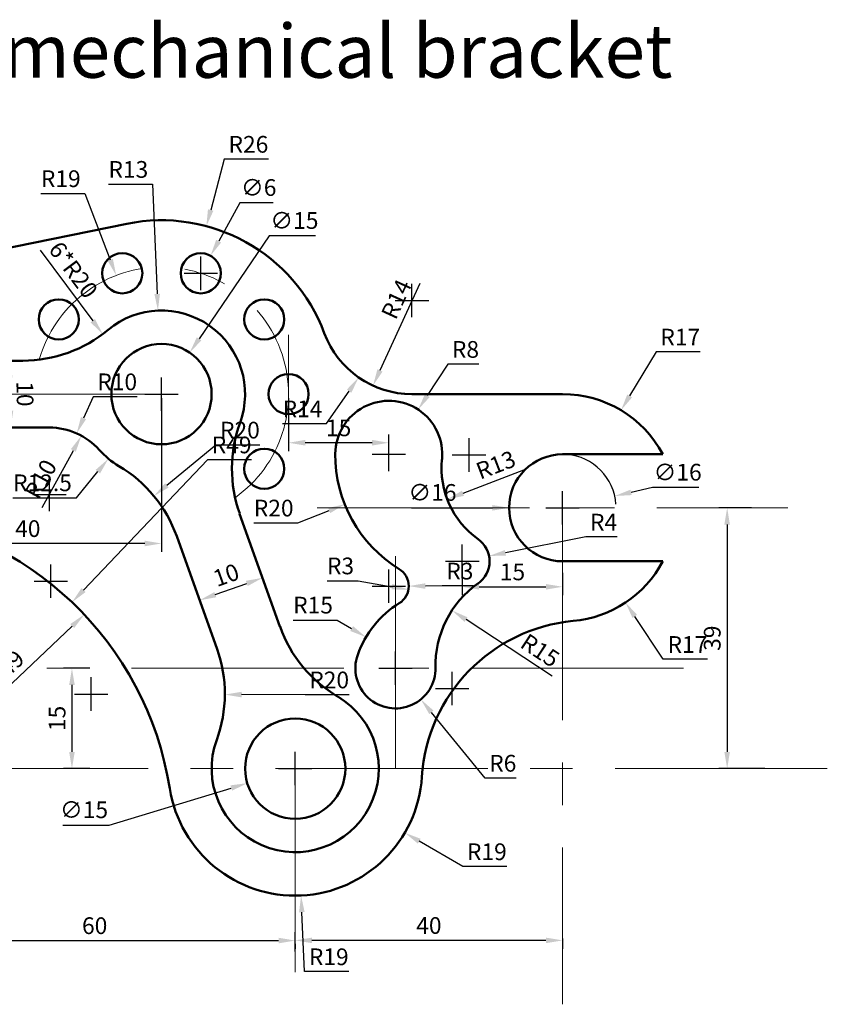
# Model space of a CAD drawing. Units: millimetres. Extents: x 59 to 241, y 36 to 183.
# Tile 2 of 2: x 120 to 241, y 36 to 183. Entities that reach past the tile are written whole.
import ezdxf

# ---------------------------------------------------------------- set-up
doc = ezdxf.new("R2010")
doc.units = ezdxf.units.MM
doc.linetypes.add('CENTER', pattern=[50.8, 31.75, -6.35, 6.35, -6.35])
for name, color, linetype, lineweight in [('M-CNTR', 1, 'CENTER', 18), ('M-DIMS', 2, 'Continuous', 25), ('M-OUTL', 7, 'Continuous', 50), ('M-TEXT', 3, 'Continuous', 25)]:
    doc.layers.add(name, color=color, linetype=linetype, lineweight=lineweight)
doc.styles.get("Standard").update_dxf_attribs({"font": 'arial.ttf'})
doc.dimstyles.new('ISO-25', dxfattribs={"dimtxt": 2.5, "dimasz": 2.5, "dimexe": 1.25, "dimexo": 0.625, "dimtad": 1, "dimtoh": 1, "dimdec": 0, "dimtxsty": 'Standard', "dimcen": 2.5, "dimadec": 0, "dimazin": 0, "dimtfac": 1, "dimtdec": 0, "dimtofl": 0, "dimtmove": 0, "dimatfit": 3, "dimfxl": 1, "dimarcsym": 0})

# ---------------------------------------------------------------- blocks, each defined once
blk = doc.blocks.new('*D2')
at = {"layer": 'Defpoints', "color": 0, "transparency": 16777216}
for p in [(101.46, 127.43), (161.46, 45.87), (161.46, 45.71)]:
    blk.add_point(p, dxfattribs=at)
at = {"layer": 'M-DIMS', "color": 0, "lineweight": -2, "transparency": 16777216}
for p, q in [((101.46, 126.8), (101.46, 44.46)), ((103.96, 45.71), (158.96, 45.71)), ((161.46, 45.24), (161.46, 44.46))]:
    blk.add_line(p, q, dxfattribs=at)
at = {"layer": 'M-DIMS', "color": 0, "transparency": 16777216}
for points in [[(103.96, 46.13), (103.96, 45.29), (101.46, 45.71)], [(158.96, 46.13), (158.96, 45.29), (161.46, 45.71)]]:
    blk.add_solid(points, dxfattribs=at)
at = {"layer": 'M-DIMS', "color": 0, "transparency": 16777216, "insert": (131.46, 47.61), "char_height": 2.5, "attachment_point": 5}
blk.add_mtext('60', dxfattribs=at)
blk = doc.blocks.new('*D3')
at = {"layer": 'Defpoints', "color": 0, "transparency": 16777216}
for p in [(161.46, 45.74), (201.46, 46.63), (161.46, 43.45)]:
    blk.add_point(p, dxfattribs=at)
at = {"layer": 'M-DIMS', "color": 0, "lineweight": -2, "transparency": 16777216}
for p, q in [((161.46, 44.07), (161.46, 46.99)), ((198.96, 45.74), (163.96, 45.74)), ((201.46, 46.01), (201.46, 44.49))]:
    blk.add_line(p, q, dxfattribs=at)
at = {"layer": 'M-DIMS', "color": 0, "transparency": 16777216}
for points in [[(163.96, 46.15), (163.96, 45.32), (161.46, 45.74)], [(198.96, 46.15), (198.96, 45.32), (201.46, 45.74)]]:
    blk.add_solid(points, dxfattribs=at)
at = {"layer": 'M-DIMS', "color": 0, "transparency": 16777216, "insert": (181.46, 47.64), "char_height": 2.5, "attachment_point": 5}
blk.add_mtext('40', dxfattribs=at)
blk = doc.blocks.new('*D4')
at = {"layer": 'Defpoints', "color": 0, "transparency": 16777216}
for p in [(209.26, 112.19), (193.65, 108.67)]:
    blk.add_point(p, dxfattribs=at)
at = {"layer": 'M-DIMS', "color": 0, "lineweight": -2, "transparency": 16777216}
for p, q in [((214.9, 113.46), (211.7, 112.73)), ((221.82, 113.46), (214.9, 113.46)), ((201.46, 107.93), (201.46, 112.93)), ((198.96, 110.43), (203.96, 110.43))]:
    blk.add_line(p, q, dxfattribs=at)
blk.add_arc((201.46, 110.43), 8, 3.7384, 85.5238, dxfattribs=at)
at = {"layer": 'M-DIMS', "color": 0, "transparency": 16777216}
blk.add_solid([(211.61, 113.14), (211.79, 112.33), (209.26, 112.19)], dxfattribs=at)
at = {"layer": 'M-DIMS', "color": 0, "transparency": 16777216, "insert": (218.67, 115.43), "char_height": 2.5, "attachment_point": 5}
blk.add_mtext('∅16', dxfattribs=at)
blk = doc.blocks.new('*D5')
at = {"layer": 'Defpoints', "color": 0, "transparency": 16777216}
for p in [(168.63, 73.61), (154.28, 69.25)]:
    blk.add_point(p, dxfattribs=at)
at = {"layer": 'M-DIMS', "color": 0, "lineweight": -2, "transparency": 16777216}
for p, q in [((161.46, 68.93), (161.46, 73.93)), ((158.96, 71.43), (163.96, 71.43)), ((133.65, 62.98), (151.89, 68.52)), ((126.71, 62.98), (133.65, 62.98))]:
    blk.add_line(p, q, dxfattribs=at)
at = {"layer": 'M-DIMS', "color": 0, "transparency": 16777216}
blk.add_solid([(151.77, 68.92), (152.01, 68.12), (154.28, 69.25)], dxfattribs=at)
at = {"layer": 'M-DIMS', "color": 0, "transparency": 16777216, "insert": (129.87, 64.95), "char_height": 2.5, "attachment_point": 5}
blk.add_mtext('∅15', dxfattribs=at)
blk = doc.blocks.new('*D6')
at = {"layer": 'Defpoints', "color": 0, "transparency": 16777216}
for p in [(148.79, 148.12), (145.87, 142.88)]:
    blk.add_point(p, dxfattribs=at)
at = {"layer": 'M-DIMS', "color": 0, "lineweight": -2, "transparency": 16777216}
for p, q in [((153.2, 156.03), (150.01, 150.3)), ((158.18, 156.03), (153.2, 156.03)), ((147.33, 143), (147.33, 148)), ((144.83, 145.5), (149.83, 145.5))]:
    blk.add_line(p, q, dxfattribs=at)
at = {"layer": 'M-DIMS', "color": 0, "transparency": 16777216}
blk.add_solid([(149.64, 150.51), (150.37, 150.1), (148.79, 148.12)], dxfattribs=at)
at = {"layer": 'M-DIMS', "color": 0, "transparency": 16777216, "insert": (156, 158), "char_height": 2.5, "attachment_point": 5}
blk.add_mtext('∅6', dxfattribs=at)
blk = doc.blocks.new('*D7')
at = {"layer": 'Defpoints', "color": 0, "transparency": 16777216}
for p in [(145.67, 133.63), (137.24, 121.23)]:
    blk.add_point(p, dxfattribs=at)
at = {"layer": 'M-DIMS', "color": 0, "lineweight": -2, "transparency": 16777216}
for p, q in [((157.55, 151.1), (147.08, 135.7)), ((164.5, 151.1), (157.55, 151.1)), ((141.46, 124.93), (141.46, 129.93)), ((138.96, 127.43), (143.96, 127.43))]:
    blk.add_line(p, q, dxfattribs=at)
at = {"layer": 'M-DIMS', "color": 0, "transparency": 16777216}
blk.add_solid([(146.74, 135.93), (147.42, 135.46), (145.67, 133.63)], dxfattribs=at)
at = {"layer": 'M-DIMS', "color": 0, "transparency": 16777216, "insert": (161.34, 153.07), "char_height": 2.5, "attachment_point": 5}
blk.add_mtext('∅15', dxfattribs=at)
blk = doc.blocks.new('*D8')
at = {"layer": 'Defpoints', "color": 0, "transparency": 16777216}
for p in [(120.69, 152.43), (132.67, 136.41)]:
    blk.add_point(p, dxfattribs=at)
at = {"layer": 'M-DIMS', "color": 0, "lineweight": -2, "transparency": 16777216}
blk.add_line((123.29, 148.95), (131.17, 138.41), dxfattribs=at)
at = {"layer": 'M-DIMS', "color": 0, "transparency": 16777216}
blk.add_solid([(131.5, 138.66), (130.84, 138.16), (132.67, 136.41)], dxfattribs=at)
at = {"layer": 'M-DIMS', "color": 0, "transparency": 16777216, "insert": (128.01, 145.82), "char_height": 2.5, "attachment_point": 5, "rotation": 306.7855}
blk.add_mtext('6*R20', dxfattribs=at)
blk = doc.blocks.new('*D11')
at = {"layer": 'Defpoints', "color": 0, "transparency": 16777216}
for p in [(129.47, 121.21), (124.69, 112.43)]:
    blk.add_point(p, dxfattribs=at)
at = {"layer": 'M-DIMS', "color": 0, "lineweight": -2, "transparency": 16777216}
blk.add_line((123.63, 110.48), (128.27, 119.02), dxfattribs=at)
at = {"layer": 'M-DIMS', "color": 0, "transparency": 16777216}
blk.add_solid([(127.91, 119.21), (128.64, 118.82), (129.47, 121.21)], dxfattribs=at)
at = {"layer": 'M-DIMS', "color": 0, "transparency": 16777216, "insert": (123.68, 114.56), "char_height": 2.5, "attachment_point": 5, "rotation": 61.439}
blk.add_mtext('R10', dxfattribs=at)
blk = doc.blocks.new('*D13')
at = {"layer": 'Defpoints', "color": 0, "transparency": 16777216}
for p in [(129.91, 94.46), (94.29, 60.81)]:
    blk.add_point(p, dxfattribs=at)
at = {"layer": 'M-DIMS', "color": 0, "lineweight": -2, "transparency": 16777216}
blk.add_line((117.07, 82.33), (128.09, 92.74), dxfattribs=at)
at = {"layer": 'M-DIMS', "color": 0, "transparency": 16777216}
blk.add_solid([(127.81, 93.05), (128.38, 92.44), (129.91, 94.46)], dxfattribs=at)
at = {"layer": 'M-DIMS', "color": 0, "transparency": 16777216, "insert": (118.39, 86.19), "char_height": 2.5, "attachment_point": 5, "rotation": 43.3695}
blk.add_mtext('R49', dxfattribs=at)
blk = doc.blocks.new('*D14')
at = {"layer": 'Defpoints', "color": 0, "transparency": 16777216}
for p in [(161.46, 71.43), (177.86, 61.83)]:
    blk.add_point(p, dxfattribs=at)
at = {"layer": 'M-DIMS', "color": 0, "lineweight": -2, "transparency": 16777216}
for p, q in [((161.46, 68.93), (161.46, 73.93)), ((158.96, 71.43), (163.96, 71.43)), ((186.52, 56.77), (180.02, 60.57)), ((193.12, 56.77), (186.52, 56.77))]:
    blk.add_line(p, q, dxfattribs=at)
at = {"layer": 'M-DIMS', "color": 0, "transparency": 16777216}
blk.add_solid([(180.23, 60.93), (179.81, 60.21), (177.86, 61.83)], dxfattribs=at)
at = {"layer": 'M-DIMS', "color": 0, "transparency": 16777216, "insert": (190.13, 58.67), "char_height": 2.5, "attachment_point": 5}
blk.add_mtext('R19', dxfattribs=at)
blk = doc.blocks.new('*D15')
at = {"layer": 'Defpoints', "color": 0, "transparency": 16777216}
for p in [(176.46, 86.43), (180.25, 81.78)]:
    blk.add_point(p, dxfattribs=at)
at = {"layer": 'M-DIMS', "color": 0, "lineweight": -2, "transparency": 16777216}
for p, q in [((176.46, 83.93), (176.46, 88.93)), ((173.96, 86.43), (178.96, 86.43)), ((189.87, 69.99), (181.83, 79.84)), ((194.52, 69.99), (189.87, 69.99))]:
    blk.add_line(p, q, dxfattribs=at)
at = {"layer": 'M-DIMS', "color": 0, "transparency": 16777216}
blk.add_solid([(182.15, 80.11), (181.51, 79.58), (180.25, 81.78)], dxfattribs=at)
at = {"layer": 'M-DIMS', "color": 0, "transparency": 16777216, "insert": (192.51, 71.9), "char_height": 2.5, "attachment_point": 5}
blk.add_mtext('R6', dxfattribs=at)
blk = doc.blocks.new('*D16')
at = {"layer": 'Defpoints', "color": 0, "transparency": 16777216}
for p in [(172.05, 91.09), (184.94, 83.42)]:
    blk.add_point(p, dxfattribs=at)
at = {"layer": 'M-DIMS', "color": 0, "lineweight": -2, "transparency": 16777216}
for p, q in [((161.14, 93.65), (167.75, 93.65)), ((167.75, 93.65), (169.9, 92.37)), ((184.94, 80.92), (184.94, 85.92)), ((182.44, 83.42), (187.44, 83.42))]:
    blk.add_line(p, q, dxfattribs=at)
at = {"layer": 'M-DIMS', "color": 0, "transparency": 16777216}
blk.add_solid([(170.11, 92.73), (169.69, 92.01), (172.05, 91.09)], dxfattribs=at)
at = {"layer": 'M-DIMS', "color": 0, "transparency": 16777216, "insert": (164.13, 95.55), "char_height": 2.5, "attachment_point": 5}
blk.add_mtext('R15', dxfattribs=at)
blk = doc.blocks.new('*D17')
at = {"layer": 'Defpoints', "color": 0, "transparency": 16777216}
for p in [(175.45, 98.71), (178.4, 98.19)]:
    blk.add_point(p, dxfattribs=at)
at = {"layer": 'M-DIMS', "color": 0, "lineweight": -2, "transparency": 16777216}
for p, q in [((166.22, 99.51), (170.88, 99.51)), ((170.88, 99.51), (175.94, 98.63))]:
    blk.add_line(p, q, dxfattribs=at)
at = {"layer": 'M-DIMS', "color": 0, "transparency": 16777216}
blk.add_solid([(176.01, 99.04), (175.87, 98.22), (178.4, 98.19)], dxfattribs=at)
at = {"layer": 'M-DIMS', "color": 0, "transparency": 16777216, "insert": (168.24, 101.41), "char_height": 2.5, "attachment_point": 5}
blk.add_mtext('R3', dxfattribs=at)
blk = doc.blocks.new('*D18')
at = {"layer": 'Defpoints', "color": 0, "transparency": 16777216}
for p in [(187.46, 118.33), (168.87, 110.95)]:
    blk.add_point(p, dxfattribs=at)
at = {"layer": 'M-DIMS', "color": 0, "lineweight": -2, "transparency": 16777216}
for p, q in [((187.46, 115.83), (187.46, 120.83)), ((184.96, 118.33), (189.96, 118.33)), ((161.85, 108.16), (166.54, 110.03)), ((155.26, 108.16), (161.85, 108.16))]:
    blk.add_line(p, q, dxfattribs=at)
at = {"layer": 'M-DIMS', "color": 0, "transparency": 16777216}
blk.add_solid([(166.39, 110.41), (166.7, 109.64), (168.87, 110.95)], dxfattribs=at)
at = {"layer": 'M-DIMS', "color": 0, "transparency": 16777216, "insert": (158.24, 110.06), "char_height": 2.5, "attachment_point": 5}
blk.add_mtext('R20', dxfattribs=at)
blk = doc.blocks.new('*D19')
at = {"layer": 'Defpoints', "color": 0, "transparency": 16777216}
for p in [(190.45, 103.22), (186.46, 102.43)]:
    blk.add_point(p, dxfattribs=at)
at = {"layer": 'M-DIMS', "color": 0, "lineweight": -2, "transparency": 16777216}
for p, q in [((204.95, 106.08), (192.9, 103.7)), ((209.6, 106.08), (204.95, 106.08)), ((186.46, 99.93), (186.46, 104.93)), ((183.96, 102.43), (188.96, 102.43))]:
    blk.add_line(p, q, dxfattribs=at)
at = {"layer": 'M-DIMS', "color": 0, "transparency": 16777216}
blk.add_solid([(192.82, 104.11), (192.98, 103.29), (190.45, 103.22)], dxfattribs=at)
at = {"layer": 'M-DIMS', "color": 0, "transparency": 16777216, "insert": (207.59, 107.96), "char_height": 2.5, "attachment_point": 5}
blk.add_mtext('R4', dxfattribs=at)
blk = doc.blocks.new('*D20')
at = {"layer": 'Defpoints', "color": 0, "transparency": 16777216}
for p in [(184.92, 95.08), (197.45, 86.85)]:
    blk.add_point(p, dxfattribs=at)
at = {"layer": 'M-DIMS', "color": 0, "lineweight": -2, "transparency": 16777216}
blk.add_line((199.9, 85.24), (187.01, 93.71), dxfattribs=at)
at = {"layer": 'M-DIMS', "color": 0, "transparency": 16777216}
blk.add_solid([(187.23, 94.06), (186.78, 93.36), (184.92, 95.08)], dxfattribs=at)
at = {"layer": 'M-DIMS', "color": 0, "transparency": 16777216, "insert": (197.92, 88.82), "char_height": 2.5, "attachment_point": 5, "rotation": 326.7033}
blk.add_mtext('R15', dxfattribs=at)
blk = doc.blocks.new('*D21')
at = {"layer": 'Defpoints', "color": 0, "transparency": 16777216}
for p in [(179.85, 125.12), (175.46, 118.43)]:
    blk.add_point(p, dxfattribs=at)
at = {"layer": 'M-DIMS', "color": 0, "lineweight": -2, "transparency": 16777216}
for p, q in [((184.29, 131.89), (181.22, 127.21)), ((188.95, 131.89), (184.29, 131.89)), ((175.46, 115.93), (175.46, 120.93)), ((172.96, 118.43), (177.96, 118.43))]:
    blk.add_line(p, q, dxfattribs=at)
at = {"layer": 'M-DIMS', "color": 0, "transparency": 16777216}
blk.add_solid([(180.87, 127.44), (181.57, 126.98), (179.85, 125.12)], dxfattribs=at)
at = {"layer": 'M-DIMS', "color": 0, "transparency": 16777216, "insert": (186.93, 133.79), "char_height": 2.5, "attachment_point": 5}
blk.add_mtext('R8', dxfattribs=at)
blk = doc.blocks.new('*D22')
at = {"layer": 'Defpoints', "color": 0, "transparency": 16777216}
for p in [(196.35, 116.34), (184.21, 111.7)]:
    blk.add_point(p, dxfattribs=at)
at = {"layer": 'M-DIMS', "color": 0, "lineweight": -2, "transparency": 16777216}
blk.add_line((195.63, 116.06), (186.54, 112.59), dxfattribs=at)
at = {"layer": 'M-DIMS', "color": 0, "transparency": 16777216}
blk.add_solid([(186.4, 112.98), (186.69, 112.21), (184.21, 111.7)], dxfattribs=at)
at = {"layer": 'M-DIMS', "color": 0, "transparency": 16777216, "insert": (191.58, 116.55), "char_height": 2.5, "attachment_point": 5, "rotation": 20.8827}
blk.add_mtext('R13', dxfattribs=at)
blk = doc.blocks.new('*D23')
at = {"layer": 'Defpoints', "color": 0, "transparency": 16777216}
for p in [(178.93, 141.43), (173.1, 128.7)]:
    blk.add_point(p, dxfattribs=at)
at = {"layer": 'M-DIMS', "color": 0, "lineweight": -2, "transparency": 16777216}
blk.add_line((180.1, 143.99), (174.14, 130.97), dxfattribs=at)
at = {"layer": 'M-DIMS', "color": 0, "transparency": 16777216}
blk.add_solid([(173.76, 131.15), (174.52, 130.8), (173.1, 128.7)], dxfattribs=at)
at = {"layer": 'M-DIMS', "color": 0, "transparency": 16777216, "insert": (176.89, 141.49), "char_height": 2.5, "attachment_point": 5, "rotation": 65.3862}
blk.add_mtext('R14', dxfattribs=at)
blk = doc.blocks.new('*D24')
at = {"layer": 'Defpoints', "color": 0, "transparency": 16777216}
for p in [(148.17, 152.55), (141.46, 127.43)]:
    blk.add_point(p, dxfattribs=at)
at = {"layer": 'M-DIMS', "color": 0, "lineweight": -2, "transparency": 16777216}
for p, q in [((150.85, 162.56), (148.82, 154.96)), ((157.44, 162.56), (150.85, 162.56)), ((141.46, 124.93), (141.46, 129.93)), ((138.96, 127.43), (143.96, 127.43))]:
    blk.add_line(p, q, dxfattribs=at)
at = {"layer": 'M-DIMS', "color": 0, "transparency": 16777216}
blk.add_solid([(148.41, 155.07), (149.22, 154.85), (148.17, 152.55)], dxfattribs=at)
at = {"layer": 'M-DIMS', "color": 0, "transparency": 16777216, "insert": (154.46, 164.46), "char_height": 2.5, "attachment_point": 5}
blk.add_mtext('R26', dxfattribs=at)
blk = doc.blocks.new('*D25')
at = {"layer": 'Defpoints', "color": 0, "transparency": 16777216}
for p in [(140.92, 139.92), (141.46, 127.43)]:
    blk.add_point(p, dxfattribs=at)
at = {"layer": 'M-DIMS', "color": 0, "lineweight": -2, "transparency": 16777216}
for p, q in [((133.51, 158.81), (140.11, 158.81)), ((140.11, 158.81), (140.81, 142.41)), ((141.46, 124.93), (141.46, 129.93)), ((138.96, 127.43), (143.96, 127.43))]:
    blk.add_line(p, q, dxfattribs=at)
at = {"layer": 'M-DIMS', "color": 0, "transparency": 16777216}
blk.add_solid([(141.23, 142.43), (140.4, 142.4), (140.92, 139.92)], dxfattribs=at)
at = {"layer": 'M-DIMS', "color": 0, "transparency": 16777216, "insert": (136.5, 160.71), "char_height": 2.5, "attachment_point": 5}
blk.add_mtext('R13', dxfattribs=at)
blk = doc.blocks.new('*D26')
at = {"layer": 'Defpoints', "color": 0, "transparency": 16777216}
for p in [(134.68, 145.18), (141.46, 127.43)]:
    blk.add_point(p, dxfattribs=at)
at = {"layer": 'M-DIMS', "color": 0, "lineweight": -2, "transparency": 16777216}
for p, q in [((123.4, 157.42), (130.01, 157.42)), ((130.01, 157.42), (133.79, 147.51)), ((141.46, 124.93), (141.46, 129.93)), ((138.96, 127.43), (143.96, 127.43))]:
    blk.add_line(p, q, dxfattribs=at)
at = {"layer": 'M-DIMS', "color": 0, "transparency": 16777216}
blk.add_solid([(134.18, 147.66), (133.4, 147.37), (134.68, 145.18)], dxfattribs=at)
at = {"layer": 'M-DIMS', "color": 0, "transparency": 16777216, "insert": (126.39, 159.32), "char_height": 2.5, "attachment_point": 5}
blk.add_mtext('R19', dxfattribs=at)
blk = doc.blocks.new('*D27')
at = {"layer": 'Defpoints', "color": 0, "transparency": 16777216}
for p in [(141.46, 127.43), (101.46, 105.09), (101.46, 101.65)]:
    blk.add_point(p, dxfattribs=at)
at = {"layer": 'M-DIMS', "color": 0, "lineweight": -2, "transparency": 16777216}
for p, q in [((141.46, 126.8), (141.46, 103.84)), ((101.46, 102.27), (101.46, 106.34)), ((138.96, 105.09), (103.96, 105.09))]:
    blk.add_line(p, q, dxfattribs=at)
at = {"layer": 'M-DIMS', "color": 0, "transparency": 16777216}
for points in [[(103.96, 105.51), (103.96, 104.68), (101.46, 105.09)], [(138.96, 105.51), (138.96, 104.68), (141.46, 105.09)]]:
    blk.add_solid(points, dxfattribs=at)
at = {"layer": 'M-DIMS', "color": 0, "transparency": 16777216, "insert": (121.46, 106.99), "char_height": 2.5, "attachment_point": 5}
blk.add_mtext('40', dxfattribs=at)
blk = doc.blocks.new('*D28')
at = {"layer": 'Defpoints', "color": 0, "transparency": 16777216}
for p in [(156.55, 100.04), (156.58, 99.96), (147.13, 96.68)]:
    blk.add_point(p, dxfattribs=at)
at = {"layer": 'M-DIMS', "color": 0, "lineweight": -2, "transparency": 16777216}
for p, q in [((149.51, 97.44), (154.22, 99.12)), ((156.76, 99.45), (157, 98.78)), ((147.34, 96.09), (147.58, 95.42))]:
    blk.add_line(p, q, dxfattribs=at)
at = {"layer": 'M-DIMS', "color": 0, "transparency": 16777216}
for points in [[(154.08, 99.51), (154.36, 98.73), (156.58, 99.96)], [(149.37, 97.83), (149.65, 97.05), (147.16, 96.6)]]:
    blk.add_solid(points, dxfattribs=at)
at = {"layer": 'M-DIMS', "color": 0, "transparency": 16777216, "insert": (151.23, 100.07), "char_height": 2.5, "attachment_point": 5, "rotation": 19.6538}
blk.add_mtext('10', dxfattribs=at)
blk = doc.blocks.new('*D29')
at = {"layer": 'Defpoints', "color": 0, "transparency": 16777216}
for p in [(118.72, 132.43), (118.9, 122.43), (118.9, 122.43)]:
    blk.add_point(p, dxfattribs=at)
at = {"layer": 'M-DIMS', "color": 0, "lineweight": -2, "transparency": 16777216}
for p, q in [((119.35, 132.44), (119.97, 132.45)), ((118.77, 129.93), (118.86, 124.93)), ((119.53, 122.44), (120.15, 122.45))]:
    blk.add_line(p, q, dxfattribs=at)
at = {"layer": 'M-DIMS', "color": 0, "transparency": 16777216}
for points in [[(119.18, 129.94), (118.35, 129.92), (118.72, 132.43)], [(119.28, 124.94), (118.44, 124.92), (118.9, 122.43)]]:
    blk.add_solid(points, dxfattribs=at)
at = {"layer": 'M-DIMS', "color": 0, "transparency": 16777216, "insert": (120.71, 127.46), "char_height": 2.5, "attachment_point": 5, "rotation": 271.0391}
blk.add_mtext('10', dxfattribs=at)
blk = doc.blocks.new('*D30')
at = {"layer": 'Defpoints', "color": 0, "transparency": 16777216}
for p in [(131.34, 86.43), (128.06, 71.43), (131.34, 71.43)]:
    blk.add_point(p, dxfattribs=at)
at = {"layer": 'M-DIMS', "color": 0, "lineweight": -2, "transparency": 16777216}
for p, q in [((130.72, 86.43), (126.81, 86.43)), ((128.06, 83.93), (128.06, 73.93)), ((130.72, 71.43), (126.81, 71.43))]:
    blk.add_line(p, q, dxfattribs=at)
at = {"layer": 'M-DIMS', "color": 0, "transparency": 16777216}
for points in [[(127.64, 83.93), (128.48, 83.93), (128.06, 86.43)], [(127.64, 73.93), (128.48, 73.93), (128.06, 71.43)]]:
    blk.add_solid(points, dxfattribs=at)
at = {"layer": 'M-DIMS', "color": 0, "transparency": 16777216, "insert": (126.16, 78.93), "char_height": 2.5, "attachment_point": 5, "rotation": 90}
blk.add_mtext('15', dxfattribs=at)
blk = doc.blocks.new('*D31')
at = {"layer": 'Defpoints', "color": 0, "transparency": 16777216}
for p in [(186.46, 102.43), (201.46, 101.33), (201.46, 98.62)]:
    blk.add_point(p, dxfattribs=at)
at = {"layer": 'M-DIMS', "color": 0, "lineweight": -2, "transparency": 16777216}
for p, q in [((186.46, 101.8), (186.46, 97.37)), ((201.46, 100.71), (201.46, 97.37)), ((188.96, 98.62), (198.96, 98.62))]:
    blk.add_line(p, q, dxfattribs=at)
at = {"layer": 'M-DIMS', "color": 0, "transparency": 16777216}
for points in [[(188.96, 99.03), (188.96, 98.2), (186.46, 98.62)], [(198.96, 99.03), (198.96, 98.2), (201.46, 98.62)]]:
    blk.add_solid(points, dxfattribs=at)
at = {"layer": 'M-DIMS', "color": 0, "transparency": 16777216, "insert": (193.96, 100.52), "char_height": 2.5, "attachment_point": 5}
blk.add_mtext('15', dxfattribs=at)
blk = doc.blocks.new('*D32')
at = {"layer": 'Defpoints', "color": 0, "transparency": 16777216}
for p in [(160.46, 127.43), (160.46, 120.16), (175.46, 118.43)]:
    blk.add_point(p, dxfattribs=at)
at = {"layer": 'M-DIMS', "color": 0, "lineweight": -2, "transparency": 16777216}
for p, q in [((160.46, 126.8), (160.46, 118.91)), ((175.46, 119.05), (175.46, 121.41)), ((172.96, 120.16), (162.96, 120.16))]:
    blk.add_line(p, q, dxfattribs=at)
at = {"layer": 'M-DIMS', "color": 0, "transparency": 16777216}
for points in [[(162.96, 120.58), (162.96, 119.74), (160.46, 120.16)], [(172.96, 120.58), (172.96, 119.74), (175.46, 120.16)]]:
    blk.add_solid(points, dxfattribs=at)
at = {"layer": 'M-DIMS', "color": 0, "transparency": 16777216, "insert": (167.96, 122.06), "char_height": 2.5, "attachment_point": 5}
blk.add_mtext('15', dxfattribs=at)
blk = doc.blocks.new('*D33')
at = {"layer": 'Defpoints', "color": 0, "transparency": 16777216}
for p in [(230.32, 110.43), (226.08, 71.43), (232.34, 71.43)]:
    blk.add_point(p, dxfattribs=at)
at = {"layer": 'M-DIMS', "color": 0, "lineweight": -2, "transparency": 16777216}
for p, q in [((229.7, 110.43), (224.83, 110.43)), ((226.08, 107.93), (226.08, 73.93)), ((231.71, 71.43), (224.83, 71.43))]:
    blk.add_line(p, q, dxfattribs=at)
at = {"layer": 'M-DIMS', "color": 0, "transparency": 16777216}
for points in [[(225.66, 107.93), (226.49, 107.93), (226.08, 110.43)], [(225.66, 73.93), (226.49, 73.93), (226.08, 71.43)]]:
    blk.add_solid(points, dxfattribs=at)
at = {"layer": 'M-DIMS', "color": 0, "transparency": 16777216, "insert": (224.17, 90.93), "char_height": 2.5, "attachment_point": 5, "rotation": 90}
blk.add_mtext('39', dxfattribs=at)
blk = doc.blocks.new('*D34')
at = {"layer": 'Defpoints', "color": 0, "transparency": 16777216}
for p in [(128.07, 96.31), (94.29, 60.81)]:
    blk.add_point(p, dxfattribs=at)
at = {"layer": 'M-DIMS', "color": 0, "lineweight": -2, "transparency": 16777216}
for p, q in [((148.34, 117.61), (129.79, 98.12)), ((154.94, 117.61), (148.34, 117.61)), ((94.29, 58.31), (94.29, 63.31)), ((91.79, 60.81), (96.79, 60.81))]:
    blk.add_line(p, q, dxfattribs=at)
at = {"layer": 'M-DIMS', "color": 0, "transparency": 16777216}
blk.add_solid([(129.49, 98.41), (130.1, 97.83), (128.07, 96.31)], dxfattribs=at)
at = {"layer": 'M-DIMS', "color": 0, "transparency": 16777216, "insert": (151.95, 119.51), "char_height": 2.5, "attachment_point": 5}
blk.add_mtext('R49', dxfattribs=at)
blk = doc.blocks.new('*D35')
at = {"layer": 'Defpoints', "color": 0, "transparency": 16777216}
for p in [(130.93, 82.58), (150.93, 82.5)]:
    blk.add_point(p, dxfattribs=at)
at = {"layer": 'M-DIMS', "color": 0, "lineweight": -2, "transparency": 16777216}
for p, q in [((130.93, 80.08), (130.93, 85.08)), ((128.43, 82.58), (133.43, 82.58)), ((162.93, 82.46), (153.43, 82.5)), ((169.52, 82.46), (162.93, 82.46))]:
    blk.add_line(p, q, dxfattribs=at)
at = {"layer": 'M-DIMS', "color": 0, "transparency": 16777216}
blk.add_solid([(153.43, 82.91), (153.43, 82.08), (150.93, 82.5)], dxfattribs=at)
at = {"layer": 'M-DIMS', "color": 0, "transparency": 16777216, "insert": (166.54, 84.36), "char_height": 2.5, "attachment_point": 5}
blk.add_mtext('R20', dxfattribs=at)
blk = doc.blocks.new('*D36')
at = {"layer": 'Defpoints', "color": 0, "transparency": 16777216}
for p in [(140.33, 112.19), (124.9, 99.46)]:
    blk.add_point(p, dxfattribs=at)
at = {"layer": 'M-DIMS', "color": 0, "lineweight": -2, "transparency": 16777216}
for p, q in [((149.59, 119.82), (142.26, 113.78)), ((156.18, 119.82), (149.59, 119.82)), ((124.9, 96.96), (124.9, 101.96)), ((122.4, 99.46), (127.4, 99.46))]:
    blk.add_line(p, q, dxfattribs=at)
at = {"layer": 'M-DIMS', "color": 0, "transparency": 16777216}
blk.add_solid([(141.99, 114.1), (142.52, 113.46), (140.33, 112.19)], dxfattribs=at)
at = {"layer": 'M-DIMS', "color": 0, "transparency": 16777216, "insert": (153.19, 121.72), "char_height": 2.5, "attachment_point": 5}
blk.add_mtext('R20', dxfattribs=at)
blk = doc.blocks.new('*D37')
at = {"layer": 'Defpoints', "color": 0, "transparency": 16777216}
for p in [(161.46, 71.43), (162.34, 52.45)]:
    blk.add_point(p, dxfattribs=at)
at = {"layer": 'M-DIMS', "color": 0, "lineweight": -2, "transparency": 16777216}
for p, q in [((161.46, 68.93), (161.46, 73.93)), ((158.96, 71.43), (163.96, 71.43)), ((162.87, 41.06), (162.45, 49.95)), ((169.47, 41.06), (162.87, 41.06))]:
    blk.add_line(p, q, dxfattribs=at)
at = {"layer": 'M-DIMS', "color": 0, "transparency": 16777216}
blk.add_solid([(162.87, 49.97), (162.04, 49.93), (162.34, 52.45)], dxfattribs=at)
at = {"layer": 'M-DIMS', "color": 0, "transparency": 16777216, "insert": (166.48, 42.96), "char_height": 2.5, "attachment_point": 5}
blk.add_mtext('R19', dxfattribs=at)
blk = doc.blocks.new('*D39')
at = {"layer": 'Defpoints', "color": 0, "transparency": 16777216}
for p in [(210.2, 125.01), (201.46, 110.43)]:
    blk.add_point(p, dxfattribs=at)
at = {"layer": 'M-DIMS', "color": 0, "lineweight": -2, "transparency": 16777216}
for p, q in [((215.45, 133.75), (211.49, 127.15)), ((222.05, 133.75), (215.45, 133.75)), ((201.46, 107.93), (201.46, 112.93)), ((198.96, 110.43), (203.96, 110.43))]:
    blk.add_line(p, q, dxfattribs=at)
at = {"layer": 'M-DIMS', "color": 0, "transparency": 16777216}
blk.add_solid([(211.13, 127.36), (211.85, 126.93), (210.2, 125.01)], dxfattribs=at)
at = {"layer": 'M-DIMS', "color": 0, "transparency": 16777216, "insert": (219.06, 135.63), "char_height": 2.5, "attachment_point": 5}
blk.add_mtext('R17', dxfattribs=at)
blk = doc.blocks.new('*D40')
at = {"layer": 'Defpoints', "color": 0, "transparency": 16777216}
for p in [(201.46, 110.43), (210.87, 96.27)]:
    blk.add_point(p, dxfattribs=at)
at = {"layer": 'M-DIMS', "color": 0, "lineweight": -2, "transparency": 16777216}
for p, q in [((201.46, 107.93), (201.46, 112.93)), ((198.96, 110.43), (203.96, 110.43)), ((216.52, 87.78), (212.26, 94.19)), ((223.12, 87.78), (216.52, 87.78))]:
    blk.add_line(p, q, dxfattribs=at)
at = {"layer": 'M-DIMS', "color": 0, "transparency": 16777216}
blk.add_solid([(212.61, 94.42), (211.91, 93.96), (210.87, 96.27)], dxfattribs=at)
at = {"layer": 'M-DIMS', "color": 0, "transparency": 16777216, "insert": (220.14, 89.66), "char_height": 2.5, "attachment_point": 5}
blk.add_mtext('R17', dxfattribs=at)
blk = doc.blocks.new('*D41')
at = {"layer": 'Defpoints', "color": 0, "transparency": 16777216}
for p in [(178.93, 141.43), (170.95, 129.93)]:
    blk.add_point(p, dxfattribs=at)
at = {"layer": 'M-DIMS', "color": 0, "lineweight": -2, "transparency": 16777216}
for p, q in [((178.93, 138.93), (178.93, 143.93)), ((176.43, 141.43), (181.43, 141.43)), ((166.16, 123.02), (169.52, 127.87)), ((159.57, 123.02), (166.16, 123.02))]:
    blk.add_line(p, q, dxfattribs=at)
at = {"layer": 'M-DIMS', "color": 0, "transparency": 16777216}
blk.add_solid([(169.18, 128.11), (169.86, 127.63), (170.95, 129.93)], dxfattribs=at)
at = {"layer": 'M-DIMS', "color": 0, "transparency": 16777216, "insert": (162.55, 124.9), "char_height": 2.5, "attachment_point": 5}
blk.add_mtext('R14', dxfattribs=at)
blk = doc.blocks.new('*D42')
at = {"layer": 'Defpoints', "color": 0, "transparency": 16777216}
for p in [(141.46, 127.43), (133.52, 117.77)]:
    blk.add_point(p, dxfattribs=at)
at = {"layer": 'M-DIMS', "color": 0, "lineweight": -2, "transparency": 16777216}
for p, q in [((141.46, 124.93), (141.46, 129.93)), ((138.96, 127.43), (143.96, 127.43)), ((128.73, 111.94), (131.94, 115.84)), ((119.2, 111.94), (128.73, 111.94))]:
    blk.add_line(p, q, dxfattribs=at)
at = {"layer": 'M-DIMS', "color": 0, "transparency": 16777216}
blk.add_solid([(131.61, 116.1), (132.26, 115.57), (133.52, 117.77)], dxfattribs=at)
at = {"layer": 'M-DIMS', "color": 0, "transparency": 16777216, "insert": (123.65, 113.84), "char_height": 2.5, "attachment_point": 5}
blk.add_mtext('R12.5', dxfattribs=at)
blk = doc.blocks.new('*D44')
at = {"layer": 'Defpoints', "color": 0, "transparency": 16777216}
for p in [(128.77, 121.56), (124.69, 112.43)]:
    blk.add_point(p, dxfattribs=at)
at = {"layer": 'M-DIMS', "color": 0, "lineweight": -2, "transparency": 16777216}
for p, q in [((131.22, 127.03), (129.79, 123.84)), ((137.81, 127.03), (131.22, 127.03)), ((124.69, 109.93), (124.69, 114.93)), ((122.19, 112.43), (127.19, 112.43))]:
    blk.add_line(p, q, dxfattribs=at)
at = {"layer": 'M-DIMS', "color": 0, "transparency": 16777216}
blk.add_solid([(129.41, 124.01), (130.17, 123.67), (128.77, 121.56)], dxfattribs=at)
at = {"layer": 'M-DIMS', "color": 0, "transparency": 16777216, "insert": (134.83, 128.94), "char_height": 2.5, "attachment_point": 5}
blk.add_mtext('R10', dxfattribs=at)
blk = doc.blocks.new('*D46')
at = {"layer": 'Defpoints', "color": 0, "transparency": 16777216}
for p in [(175.45, 98.71), (178.45, 98.72)]:
    blk.add_point(p, dxfattribs=at)
at = {"layer": 'M-DIMS', "color": 0, "lineweight": -2, "transparency": 16777216}
for p, q in [((175.45, 96.21), (175.45, 101.21)), ((172.95, 98.71), (177.95, 98.71)), ((183.45, 98.74), (180.95, 98.73)), ((188.1, 98.74), (183.45, 98.74))]:
    blk.add_line(p, q, dxfattribs=at)
at = {"layer": 'M-DIMS', "color": 0, "transparency": 16777216}
blk.add_solid([(180.95, 99.15), (180.95, 98.31), (178.45, 98.72)], dxfattribs=at)
at = {"layer": 'M-DIMS', "color": 0, "transparency": 16777216, "insert": (186.09, 100.64), "char_height": 2.5, "attachment_point": 5}
blk.add_mtext('R3', dxfattribs=at)
blk = doc.blocks.new('*D47')
at = {"layer": 'Defpoints', "color": 0, "transparency": 16777216}
for p in [(193.46, 110.43), (209.46, 110.43)]:
    blk.add_point(p, dxfattribs=at)
at = {"layer": 'M-DIMS', "color": 0, "lineweight": -2, "transparency": 16777216}
for p, q in [((201.46, 107.93), (201.46, 112.93)), ((178.84, 110.43), (185.77, 110.43)), ((185.77, 110.43), (190.96, 110.43)), ((198.96, 110.43), (203.96, 110.43))]:
    blk.add_line(p, q, dxfattribs=at)
at = {"layer": 'M-DIMS', "color": 0, "transparency": 16777216}
blk.add_solid([(190.96, 110.84), (190.96, 110.01), (193.46, 110.43)], dxfattribs=at)
at = {"layer": 'M-DIMS', "color": 0, "transparency": 16777216, "insert": (181.99, 112.4), "char_height": 2.5, "attachment_point": 5}
blk.add_mtext('∅16', dxfattribs=at)

msp = doc.modelspace()

# ---------------------------------------------------------------- linework, layer by layer
at = {"layer": 'M-CNTR'}
for p, q in [((160.46, 127.43), (160.46, 136.28)), ((141.46, 127.43), (69.53, 127.43)), ((164.75, 110.43), (235.16, 110.43)), ((201.46, 110.43), (201.46, 36.18)), ((176.46, 71.43), (176.46, 104.6)), ((219.53, 86.43), (115.15, 86.43)), ((241.06, 71.43), (65.85, 71.43)), ((161.46, 71.43), (161.46, 40.98))]:
    msp.add_line(p, q, dxfattribs=at)
msp.add_arc((141.46, 127.43), 19, 305.394, 164.2598, dxfattribs=at)
at = {"layer": 'M-OUTL'}
for p, q in [((136.26, 152.9), (97.86, 145.06)), ((113.12, 132.43), (120.69, 132.43)), ((201.46, 127.43), (178.93, 127.43)), ((113.12, 122.43), (124.69, 122.43)), ((201.46, 118.43), (216.46, 118.43)), ((153.15, 109.55), (159.18, 92.67)), ((143.73, 106.19), (149.77, 89.3)), ((201.46, 102.43), (216.46, 102.43))]:
    msp.add_line(p, q, dxfattribs=at)
for centre, radius in [((135.59, 145.5), 3), ((147.33, 145.5), 3), ((126.09, 138.6), 3), ((156.83, 138.6), 3), ((141.46, 127.43), 7.5), ((160.46, 127.43), 3), ((156.83, 116.26), 3), ((161.46, 71.43), 7.5)]:
    msp.add_circle(centre, radius, dxfattribs=at)
for centre, radius, start, end in [((141.46, 127.43), 26, 20.4873, 101.537), ((141.46, 127.43), 12.5, 339.9387, 129.7151), ((120.69, 152.43), 20, 270, 309.7151), ((178.93, 141.43), 14, 200.4873, 270), ((201.46, 110.43), 17, 28.0725, 90), ((175.46, 118.43), 8, 354.2856, 179.5159), ((124.69, 112.43), 10, 41.8103, 90), ((171.99, 116.28), 20, 159.9387, 199.6538), ((141.46, 127.43), 12.5, 221.8103, 239.369), ((187.46, 118.33), 20, 179.5159, 238.5198), ((201.46, 110.43), 8, 90, 270), ((124.9, 99.46), 20, 19.6538, 59.369), ((196.35, 116.34), 13, 174.2856, 234.5699), ((94.29, 60.81), 49, 8.9813, 83.8599), ((186.46, 102.43), 4.07, 305.2119, 54.5699), ((201.46, 110.43), 17, 275.3413, 331.9275), ((175.45, 98.71), 3, 301.8293, 58.5198), ((197.45, 86.85), 15, 125.2119, 181.602), ((184.94, 83.42), 15, 121.8293, 160.4648), ((205.37, 68.61), 25, 95.3413, 176.3284), ((178.02, 99.39), 20, 199.6538, 239.369), ((130.93, 82.58), 20, 339.9387, 19.6538), ((176.46, 86.43), 6, 160.4648, 1.1442), ((161.46, 71.43), 12.5, 159.9387, 59.369), ((161.46, 71.43), 19, 188.9813, 356.3284)]:
    msp.add_arc(centre, radius, start, end, dxfattribs=at)

# ---------------------------------------------------------------- texts
at = {"layer": 'M-TEXT', "insert": (71.54, 182.74), "char_height": 8, "attachment_point": 1}
msp.add_mtext_dynamic_manual_height_columns('complex mechanical bracket', width=206.9654, gutter_width=12.5, heights=[0], dxfattribs=at)

# ---------------------------------------------------------------- dimensions: what is measured, and where the dimension line sits
at = {"layer": 'M-DIMS'}
for center, mpoint, override, picture, middle in [((141.46, 127.43), (148.17, 152.55), {"dimclrd": 0, "dimclre": 0, "dimclrt": 0}, '*D24', (154.46, 162.56)), ((141.46, 127.43), (140.92, 139.92), {"dimclrd": 0, "dimclre": 0, "dimclrt": 0}, '*D25', (136.5, 158.81)), ((141.46, 127.43), (134.68, 145.18), {"dimclrd": 0, "dimclre": 0, "dimclrt": 0}, '*D26', (126.39, 157.42)), ((178.93, 141.43), (173.1, 128.7), {"dimclrd": 0, "dimclre": 0, "dimclrt": 0}, '*D23', (178.6, 140.71)), ((178.93, 141.43), (170.95, 129.93), {"dimdec": 0, "dimlfac": 1, "dimrnd": 0, "dimzin": 0, "dimdsep": 46, "dimlunit": 2}, '*D41', (162.55, 123.02)), ((201.46, 110.43), (210.2, 125.01), {"dimdec": 0, "dimlfac": 1, "dimrnd": 0, "dimzin": 0, "dimdsep": 46, "dimlunit": 2}, '*D39', (219.06, 133.75)), ((175.46, 118.43), (179.85, 125.12), {"dimclrd": 0, "dimclre": 0, "dimclrt": 0}, '*D21', (186.93, 131.89)), ((124.69, 112.43), (128.77, 121.56), {"dimdec": 0, "dimlfac": 1, "dimrnd": 0, "dimzin": 0, "dimdsep": 46, "dimlunit": 2}, '*D44', (134.83, 127.03)), ((124.9, 99.46), (140.33, 112.19), {"dimdec": 0, "dimlfac": 1, "dimrnd": 0, "dimzin": 0, "dimdsep": 46, "dimlunit": 2}, '*D36', (153.19, 119.82)), ((94.29, 60.81), (128.07, 96.31), {"dimdec": 0, "dimlfac": 1, "dimrnd": 0, "dimzin": 0, "dimdsep": 46, "dimlunit": 2}, '*D34', (151.95, 117.61)), ((124.69, 112.43), (129.47, 121.21), {"dimclrd": 0, "dimclre": 0, "dimclrt": 0}, '*D11', (125.35, 113.65)), ((196.35, 116.34), (184.21, 111.7), {"dimclrd": 0, "dimclre": 0, "dimclrt": 0}, '*D22', (192.25, 114.77)), ((201.46, 110.43), (210.87, 96.27), {"dimdec": 0, "dimlfac": 1, "dimrnd": 0, "dimzin": 0, "dimdsep": 46, "dimlunit": 2}, '*D40', (220.14, 87.78)), ((186.46, 102.43), (190.45, 103.22), {"dimclrd": 0, "dimclre": 0, "dimclrt": 0}, '*D19', (204.95, 106.08)), ((175.45, 98.71), (178.4, 98.19), {"dimclrd": 0, "dimclre": 0, "dimclrt": 0}, '*D17', (170.88, 99.51)), ((94.29, 60.81), (129.91, 94.46), {"dimclrd": 0, "dimclre": 0, "dimclrt": 0}, '*D13', (119.7, 84.81)), ((197.45, 86.85), (184.92, 95.08), {"dimclrd": 0, "dimclre": 0, "dimclrt": 0}, '*D20', (196.87, 87.23)), ((176.46, 86.43), (180.25, 81.78), {"dimclrd": 0, "dimclre": 0, "dimclrt": 0}, '*D15', (192.51, 69.99)), ((130.93, 82.58), (150.93, 82.5), {"dimdec": 0, "dimlfac": 1, "dimrnd": 0, "dimzin": 0, "dimdsep": 46, "dimlunit": 2}, '*D35', (162.93, 82.46)), ((161.46, 71.43), (177.86, 61.83), {"dimclrd": 0, "dimclre": 0, "dimclrt": 0}, '*D14', (190.13, 56.77)), ((161.46, 71.43), (162.34, 52.45), {"dimdec": 0, "dimlfac": 1, "dimrnd": 0, "dimzin": 0, "dimdsep": 46, "dimlunit": 2}, '*D37', (166.48, 41.06))]:
    dim = msp.add_radius_dim(center=center, mpoint=mpoint, dimstyle='ISO-25', override=override, dxfattribs=at)
    dim.commit()
    dim.dimension.update_dxf_attribs({"geometry": picture, "text_midpoint": middle, "dimtype": 164})
for p1, p2, picture, middle in [((145.87, 142.88), (148.79, 148.12), '*D6', (156, 156.03)), ((137.24, 121.23), (145.67, 133.63), '*D7', (161.34, 151.1)), ((193.65, 108.67), (209.26, 112.19), '*D4', (214.9, 113.46)), ((168.63, 73.61), (154.28, 69.25), '*D5', (129.87, 62.98))]:
    dim = msp.add_diameter_dim_2p(p1=p1, p2=p2, dimstyle='ISO-25', override={"dimclrd": 0, "dimclre": 0, "dimclrt": 0}, dxfattribs=at)
    dim.commit()
    dim.dimension.update_dxf_attribs({"geometry": picture, "text_midpoint": middle, "dimtype": 163})
dim = msp.add_radius_dim(center=(120.69, 152.43), mpoint=(132.67, 136.41), text='6*<>', dimstyle='ISO-25', override={"dimclrd": 0, "dimclre": 0, "dimclrt": 0}, dxfattribs=at)
dim.commit()
dim.dimension.update_dxf_attribs({"geometry": '*D8', "text_midpoint": (126.48, 144.68), "dimtype": 164})
for p1, p2, distance, picture, middle in [((118.72, 132.43), (118.9, 122.43), 0, '*D29', (120.71, 127.46)), ((147.13, 96.68), (156.55, 100.04), -0.08, '*D28', (151.23, 100.07))]:
    dim = msp.add_aligned_dim(p1=p1, p2=p2, distance=distance, dimstyle='ISO-25', override={"dimclrd": 0, "dimclre": 0, "dimclrt": 0}, dxfattribs=at)
    dim.commit()
    dim.dimension.update_dxf_attribs({"geometry": picture, "text_midpoint": middle})
for center, mpoint, override, picture, middle in [((141.46, 127.43), (133.52, 117.77), {"dimdec": 1, "dimlfac": 1, "dimrnd": 0, "dimzin": 0, "dimdsep": 46, "dimlunit": 2}, '*D42', (123.65, 113.84)), ((187.46, 118.33), (168.87, 110.95), {"dimclrd": 0, "dimclre": 0, "dimclrt": 0}, '*D18', (158.24, 110.06)), ((175.45, 98.71), (178.45, 98.72), {"dimdec": 0, "dimlfac": 1, "dimrnd": 0, "dimzin": 0, "dimdsep": 46, "dimlunit": 2}, '*D46', (186.09, 100.64)), ((184.94, 83.42), (172.05, 91.09), {"dimclrd": 0, "dimclre": 0, "dimclrt": 0}, '*D16', (164.13, 95.55))]:
    dim = msp.add_radius_dim(center=center, mpoint=mpoint, dimstyle='ISO-25', override=override, dxfattribs=at)
    dim.commit()
    dim.dimension.update_dxf_attribs({"geometry": picture, "text_midpoint": middle})
for base, p1, p2, picture, middle in [((161.46, 45.71), (101.46, 127.43), (161.46, 45.87), '*D2', (131.46, 47.61)), ((101.46, 105.09), (141.46, 127.43), (101.46, 101.65), '*D27', (121.46, 106.99)), ((160.46, 120.16), (175.46, 118.43), (160.46, 127.43), '*D32', (167.96, 122.06)), ((201.46, 98.62), (186.46, 102.43), (201.46, 101.33), '*D31', (193.96, 100.52)), ((161.46, 45.74), (201.46, 46.63), (161.46, 43.45), '*D3', (181.46, 47.64))]:
    dim = msp.add_linear_dim(base=base, p1=p1, p2=p2, dimstyle='ISO-25', override={"dimclrd": 0, "dimclre": 0, "dimclrt": 0}, dxfattribs=at)
    dim.commit()
    dim.dimension.update_dxf_attribs({"geometry": picture, "text_midpoint": middle})
dim = msp.add_diameter_dim_2p(p1=(209.46, 110.43), p2=(193.46, 110.43), dimstyle='ISO-25', override={"dimdec": 0, "dimlfac": 1, "dimrnd": 0, "dimzin": 0, "dimdsep": 46, "dimlunit": 2}, dxfattribs=at)
dim.commit()
dim.dimension.update_dxf_attribs({"geometry": '*D47', "text_midpoint": (185.77, 110.43)})
for base, p1, p2, picture, middle in [((226.08, 71.43), (230.32, 110.43), (232.34, 71.43), '*D33', (224.17, 90.93)), ((128.06, 71.43), (131.34, 86.43), (131.34, 71.43), '*D30', (126.16, 78.93))]:
    dim = msp.add_linear_dim(base=base, p1=p1, p2=p2, angle=90, dimstyle='ISO-25', override={"dimclrd": 0, "dimclre": 0, "dimclrt": 0}, dxfattribs=at)
    dim.commit()
    dim.dimension.update_dxf_attribs({"geometry": picture, "text_midpoint": middle})

doc.saveas('drawing.dxf')
